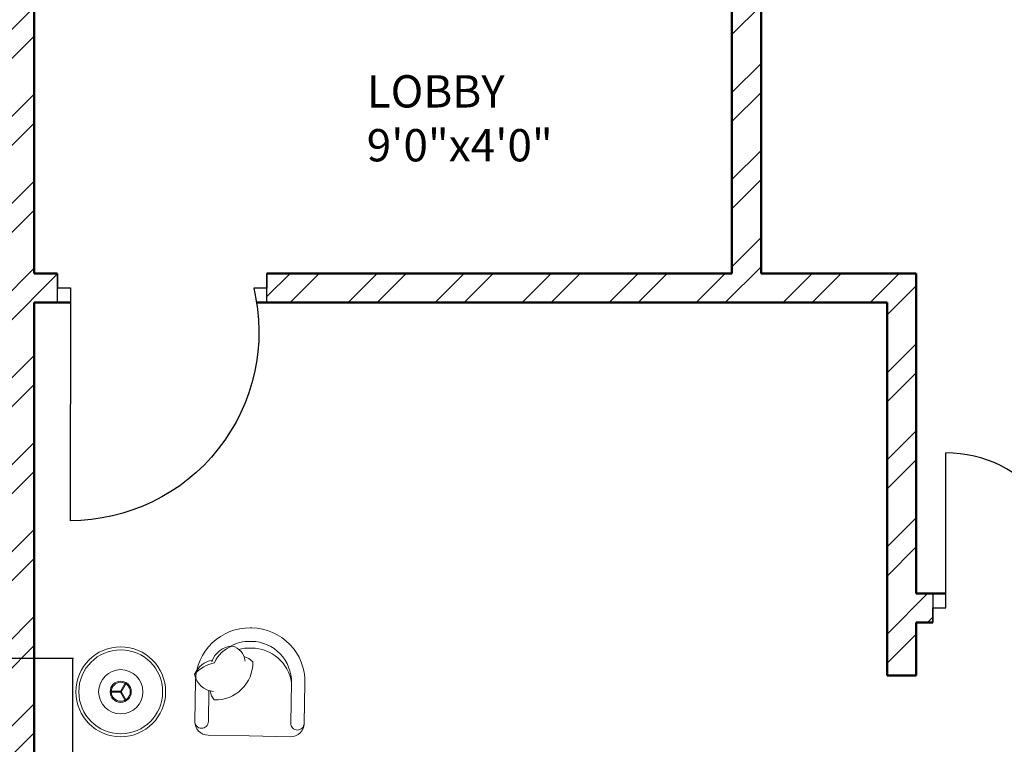
# Model space of a CAD drawing. Units: inches. Extents: x 963 to 2075, y 289 to 2657.
# Tile 54 of 98: x 1511 to 1663, y 1803 to 1915. Entities that reach past the tile are written whole.
import ezdxf

# ---------------------------------------------------------------- set-up
doc = ezdxf.new("R2010")
doc.units = ezdxf.units.IN
for name, color, linetype, lineweight in [('A-ANNO-DIMS', 2, 'Continuous', 18), ('A-AREA-IDEN', 7, 'Continuous', 18), ('A-DOOR', 4, 'Continuous', 25), ('A-FURN', 8, 'Continuous', 18), ('A-WALL', 7, 'Continuous', 50), ('A-WALL-PATT', 8, 'Continuous', 13)]:
    doc.layers.add(name, color=color, linetype=linetype, lineweight=lineweight)
doc.styles.get("Standard").update_dxf_attribs({"font": 'arial.ttf'})
doc.dimstyles.get("Standard").update_dxf_attribs({"dimtxt": 0.18, "dimasz": 0.18, "dimexe": 0.18, "dimexo": 0.0625, "dimgap": 0.09, "dimtad": 0, "dimtih": 1, "dimtoh": 1, "dimdec": 4, "dimzin": 0, "dimdsep": 46, "dimtxsty": 'Standard', "dimcen": 0.09, "dimadec": 0, "dimazin": 0, "dimtfac": 1, "dimtdec": 4, "dimtofl": 0, "dimtmove": 0, "dimatfit": 3, "dimfxl": 1, "dimtolj": 1, "dimtzin": 0, "dimarcsym": 0})

# ---------------------------------------------------------------- blocks, each defined once
blk = doc.blocks.new('ARMCHAIR-B')
at = {"ltscale": 0.03}
blk.add_lwpolyline([(8.89, -0.24), (2.51, -0.24, -0.414214), (0.42, 1.85), (0.42, 8.12, -0.414214), (8.78, 16.48), (8.89, 16.48), (8.99, 16.48, -0.414214), (17.35, 8.12), (17.35, 1.85, -0.414214), (15.26, -0.24), (8.89, -0.24)], format="xyb", dxfattribs=at)
for points in [[(2.51, 8.12, -0.414214), (8.78, 14.39), (8.89, 14.39)], [(12.1, 13.56, 0.130591), (8.99, 14.39), (8.89, 14.39)], [(2.51, 8.12, -0.372719), (8.78, 13.35), (8.89, 13.35)], [(10.77, 13.12, 0.072384), (8.99, 13.35), (8.89, 13.35)], [(14.89, 11.12, 0.306663), (11.77, 13.61, 0.30633), (9.74, 11.33, -0.872847)], [(17.52, 9.18, 0.14773), (14.47, 10.97, 0.213343), (11.77, 13.61, 0.178662)], [(15.05, 6.61, -0.165541), (14.41, 5.23, -0.425989), (8.54, 11.21, -0.121523), (9.93, 12.04, 7.115464)], [(14.53, 6.54, 0.356772), (17.52, 9.18, 0.249542), (14.81, 11.35, -9.61688)], [(2.51, 8.12), (2.51, 1.85, -0.414214), (1.47, 0.81), (1.47, 0.81, -0.414214), (0.42, 1.85)], [(15.26, 6.66), (15.26, 1.85, 0.414214), (16.31, 0.81), (16.31, 0.81, 0.414214), (17.35, 1.85)]]:
    blk.add_lwpolyline(points, format="xyb")
blk = doc.blocks.new('DOOR-3')
for p, q in [((2, 2.25), (2, 38.25)), ((0, 4.5), (0, 0)), ((32.39, 4.5), (32.39, 0)), ((0, 0), (0, 2.25)), ((0, 2.25), (2, 2.25)), ((32.39, 2.25), (30.39, 2.25)), ((32.39, 0), (32.39, 2.25))]:
    blk.add_line(p, q)
blk.add_arc((2, 9.06), 29.19, 346.5105, 90)
blk = doc.blocks.new('*D28')
at = {"layer": 'A-ANNO-DIMS', "color": 0, "lineweight": -2, "transparency": 16777216}
for p, q in [((1506.73, 1816.32), (1519.01, 1816.32)), ((1518.83, 1816.14), (1518.83, 1775.94)), ((1518.83, 1735.38), (1518.83, 1775.58)), ((1506.73, 1735.2), (1519.01, 1735.2))]:
    blk.add_line(p, q, dxfattribs=at)
at = {"layer": 'A-ANNO-DIMS', "color": 0, "transparency": 16777216}
for points in [[(1518.8, 1816.14), (1518.86, 1816.14), (1518.83, 1816.32)], [(1518.8, 1735.38), (1518.86, 1735.38), (1518.83, 1735.2)]]:
    blk.add_solid(points, dxfattribs=at)
at = {"layer": 'Defpoints', "color": 0, "transparency": 16777216}
for p in [(1506.66, 1816.32), (1518.83, 1816.32), (1506.66, 1735.2)]:
    blk.add_point(p, dxfattribs=at)
at = {"layer": 'A-ANNO-DIMS', "color": 0, "transparency": 16777216, "insert": (1518.83, 1775.76), "char_height": 0.18, "attachment_point": 5}
blk.add_mtext('\\A1;3-SEAT SOFA 81 TYP.', dxfattribs=at)

msp = doc.modelspace()

# ---------------------------------------------------------------- hatches: boundary and pattern name
at = {"layer": 'A-WALL-PATT'}
h = msp.add_hatch(dxfattribs=at)
h.set_pattern_fill('ANSI32', color=256)
h.paths.add_polyline_path([(1473.61, 2163.07), (1473.61, 2165.32), (1376.42, 2165.32), (1376.42, 2227.98), (1371.92, 2227.98), (1371.92, 2214.82), (1368.41, 2214.82), (1368.41, 2210.32), (1371.92, 2210.32), (1371.92, 2160.82), (1395.92, 2160.82), (1395.92, 2090.32), (1217.34, 2090.32), (1217.34, 2085.82), (1395.92, 2085.82), (1458.92, 2085.82), (1458.92, 2108.32), (1454.42, 2108.32), (1454.42, 2090.32), (1400.42, 2090.32), (1400.42, 2160.82), (1473.61, 2160.82)])
h.paths.add_polyline_path([(1649.42, 2210.32), (1653.23, 2210.32), (1653.23, 2214.82), (1649.42, 2214.82), (1649.42, 2227.98), (1644.92, 2227.98), (1644.92, 2165.32), (1550.1, 2165.32), (1550.1, 2160.82), (1620.92, 2160.82), (1620.92, 2112.82), (1555.45, 2112.82), (1555.45, 2108.32), (1584.33, 2108.32), (1584.33, 2084.92), (1588.83, 2084.92), (1588.83, 2108.32), (1625.42, 2108.32), (1667.95, 2108.32), (1667.95, 2022.67), (1588.83, 2022.67), (1588.83, 2047.41), (1584.33, 2047.41), (1584.33, 1996), (1588.83, 1996), (1588.83, 2018.32), (1667.95, 2018.17), (1667.95, 1928.32), (1625.42, 1928.32), (1625.42, 1923.82), (1672.45, 1923.82), (1672.45, 1928.32), (1672.45, 1946.66), (1785.45, 1946.66), (1785.45, 1951.16), (1743.03, 1951.16), (1743.03, 2017.92), (1841.42, 2017.92), (1841.42, 2014.77), (1845.92, 2014.77), (1845.92, 2017.92), (1905.92, 2017.92), (1905.92, 1987.51), (1910.42, 1987.51), (1910.42, 2022.42), (1910.42, 2068.52), (1905.92, 2068.52), (1905.92, 2022.42), (1845.92, 2022.42), (1845.92, 2025.85), (1843.67, 2025.85), (1841.42, 2025.85), (1841.42, 2022.42), (1743.03, 2022.42), (1743.03, 2084.03), (1768.45, 2084.03), (1785.45, 2084.03), (1785.45, 2088.53), (1672.45, 2088.53), (1672.45, 2112.82), (1667.95, 2112.82), (1625.42, 2112.82), (1625.42, 2160.82), (1649.42, 2160.82)])
h.paths.add_polyline_path([(1672.45, 2084.03), (1738.53, 2084.03), (1738.53, 1951.16), (1672.45, 1951.16)], flags=16)
h.paths.add_polyline_path([(1672.45, 2084.03), (1738.53, 2084.03), (1705.49, 2017.6)], flags=0)
h.paths.add_polyline_path([(1262.77, 2085.82), (1258.27, 2085.82), (1258.27, 2023.28), (1184.42, 2023.28), (1184.42, 2018.78), (1258.27, 2018.78), (1258.27, 1950.82), (1262.77, 1950.82)])
h.paths.add_polyline_path([(1312.27, 2085.82), (1307.77, 2085.82), (1307.77, 1950.82), (1312.27, 1950.82)])
h.paths.add_polyline_path([(1458.92, 1950.82), (1395.92, 1950.82), (1216.57, 1950.82), (1216.57, 1946.32), (1346.42, 1946.32), (1395.92, 1946.32), (1395.92, 1875.82), (1371.92, 1875.82), (1371.92, 1826.32), (1368.93, 1826.32), (1368.93, 1821.82), (1371.92, 1821.82), (1371.92, 1813.62), (1376.42, 1813.62), (1376.42, 1871.32), (1474.5, 1871.32), (1474.5, 1873.57), (1474.5, 1875.82), (1400.42, 1875.82), (1400.42, 1946.32), (1454.42, 1946.32), (1454.42, 1928.32), (1458.92, 1928.32)])
h.paths.add_polyline_path([(1184.42, 2120.78), (1167.92, 2120.78), (1167.92, 2134.81), (1165.67, 2134.81), (1163.42, 2134.81), (1163.42, 2120.78), (1119.92, 2120.78), (1119.92, 2098.1), (1124.42, 2098.1), (1124.42, 2116.28), (1167.92, 2116.28), (1179.92, 2116.28), (1179.92, 2045.92), (1184.42, 2045.92), (1184.42, 2090.32), (1184.42, 2116.28)])
h.paths.add_polyline_path([(1124.42, 2018.78), (1179.92, 2018.78), (1179.92, 2016.29), (1184.42, 2016.29), (1184.42, 2023.28), (1184.42, 2026.59), (1182.17, 2026.59), (1179.92, 2026.59), (1179.92, 2023.28), (1124.42, 2023.28), (1124.42, 2074.1), (1119.92, 2074.1), (1119.92, 2018.78), (1119.92, 1979.63), (1124.42, 1979.63)])
h.paths.add_polyline_path([(1184.42, 1925.78), (1184.42, 1946.32), (1184.42, 1996.07), (1182.17, 1996.07), (1179.92, 1996.07), (1179.92, 1925.78), (1124.42, 1925.78), (1124.42, 1955.63), (1119.92, 1955.5), (1119.92, 1921.28), (1158.92, 1921.28), (1158.92, 1909.98), (1163.42, 1909.98), (1163.42, 1921.28), (1184.42, 1921.28)])
h.paths.add_polyline_path([(1341.45, 1826.32), (1163.42, 1826.32), (1163.42, 1849.98), (1158.92, 1849.98), (1158.92, 1821.82), (1158.92, 1804.03), (1163.42, 1804.03), (1163.42, 1821.82), (1341.45, 1821.82)])
h.paths.add_polyline_path([(1222.98, 1713.82), (1163.42, 1713.82), (1163.42, 1744.03), (1161.17, 1744.03), (1158.92, 1744.03), (1158.92, 1713.82), (1119.92, 1713.82), (1119.92, 1694.65), (1124.42, 1694.65), (1124.42, 1709.32), (1158.92, 1709.32), (1222.98, 1709.32)])
h.paths.add_polyline_path([(1328.42, 1713.82), (1252.04, 1713.82), (1252.04, 1711.57), (1252.04, 1709.32), (1256.42, 1709.32), (1256.42, 1547.32), (1232.94, 1547.32), (1232.94, 1545.07), (1232.94, 1542.82), (1292.42, 1542.82), (1292.42, 1527.63), (1296.92, 1527.63), (1296.92, 1542.82), (1299.46, 1542.82), (1299.46, 1547.32), (1260.92, 1547.32), (1260.92, 1658.32), (1343.66, 1658.32), (1343.66, 1660.57), (1343.66, 1662.82), (1328.42, 1662.82), (1328.42, 1676.59), (1327.4, 1676.59), (1323.92, 1676.59), (1323.92, 1662.82), (1260.92, 1662.82), (1260.92, 1709.32), (1323.92, 1709.32), (1323.92, 1699.85), (1328.42, 1699.85)])
h.paths.add_polyline_path([(1649.42, 1875.82), (1625.42, 1875.82), (1625.42, 1928.32), (1620.92, 1928.32), (1588.83, 1928.32), (1588.83, 1950.59), (1584.33, 1950.59), (1584.33, 1928.32), (1555.45, 1928.32), (1555.45, 1923.82), (1620.92, 1923.82), (1620.92, 1875.82), (1548.95, 1875.82), (1548.95, 1873.57), (1548.95, 1871.32), (1644.92, 1871.32), (1644.92, 1813.62), (1649.42, 1813.62), (1649.42, 1821.82), (1652.04, 1821.82), (1652.04, 1824.07), (1652.04, 1826.32), (1649.42, 1826.32)])
h.paths.add_polyline_path([(1512.92, 1871.32), (1516.48, 1871.32), (1516.48, 1875.82), (1512.92, 1875.82), (1512.92, 1923.82), (1512.92, 1928.32), (1512.92, 1930.83), (1508.42, 1930.83), (1508.42, 1875.82), (1504.41, 1875.82), (1504.41, 1871.32), (1508.42, 1871.32), (1508.42, 1713.82), (1376.42, 1713.82), (1376.42, 1743.32), (1371.92, 1743.32), (1371.92, 1709.32), (1371.92, 1706.01), (1376.42, 1706.01), (1376.42, 1709.32), (1508.42, 1709.32), (1508.42, 1547.32), (1501.87, 1547.32), (1501.87, 1542.82), (1508.42, 1542.82), (1508.42, 1482.82), (1508.42, 1436.32), (1512.92, 1436.32), (1512.92, 1542.82), (1519.32, 1542.82), (1519.32, 1545.07), (1519.32, 1547.32), (1512.92, 1547.32), (1512.92, 1709.32), (1644.92, 1709.32), (1644.92, 1707.55), (1649.42, 1707.55), (1649.42, 1709.32), (1649.42, 1743.32), (1644.92, 1743.32), (1644.92, 1713.82), (1512.92, 1713.82)])
h.paths.add_polyline_path([(1129.88, 1545.07), (1129.88, 1547.32), (1124.42, 1547.32), (1095.92, 1547.32), (1095.92, 1614.82), (1124.42, 1614.82), (1124.42, 1619.32), (1095.92, 1619.32), (1091.42, 1619.32), (1091.42, 1542.82), (1095.92, 1542.82), (1119.92, 1542.82), (1129.88, 1542.82)])
h.paths.add_polyline_path([(1208.42, 1542.82), (1211.74, 1542.82), (1211.74, 1547.32), (1198.85, 1547.32), (1198.85, 1542.82), (1203.92, 1542.82), (1203.92, 1478.32), (1208.42, 1478.32), (1296.92, 1478.32), (1296.92, 1503.63), (1292.42, 1503.63), (1292.42, 1482.82), (1208.42, 1482.82)])
h.paths.add_polyline_path([(1430.42, 1542.82), (1435.7, 1542.82), (1435.7, 1545.07), (1435.7, 1547.32), (1422.66, 1547.32), (1422.66, 1545.07), (1422.66, 1542.82), (1425.92, 1542.82), (1425.92, 1482.86), (1341.92, 1482.86), (1341.92, 1502.73), (1337.42, 1502.73), (1337.42, 1478.36), (1425.92, 1478.36), (1425.92, 1440.82), (1425.92, 1436.32), (1430.42, 1436.32)])
h.paths.add_polyline_path([(1698.48, 2004.26), (1727.69, 2004.26), (1727.69, 2022.92), (1698.48, 2022.92)], flags=8)

# ---------------------------------------------------------------- linework, layer by layer
at = {"layer": 'A-DOOR'}
for p, q in [((1654.04, 1824.07), (1654.04, 1848.07)), ((1652.04, 1826.32), (1652.04, 1821.82)), ((1652.04, 1821.82), (1652.04, 1824.07)), ((1652.04, 1824.07), (1654.04, 1824.07))]:
    msp.add_line(p, q, dxfattribs=at)
msp.add_arc((1654.04, 1828.99), 19.08, 345.0651, 90, dxfattribs=at)
at = {"layer": 'A-FURN', "ltscale": 0.03}
for p, q in [((1526.25, 1811.15), (1527.07, 1812.56)), ((1526.38, 1811.07), (1527.19, 1812.49)), ((1526.31, 1811.18), (1524.68, 1811.18)), ((1526.31, 1811.04), (1524.68, 1811.04)), ((1526.25, 1811.07), (1527.07, 1809.66)), ((1526.38, 1811.15), (1527.19, 1809.73))]:
    msp.add_line(p, q, dxfattribs=at)
for radius in [6.95, 3.42, 1.64, 1.47]:
    msp.add_circle((1526.31, 1811.11), radius, dxfattribs=at)
at = {"layer": 'A-FURN'}
msp.add_circle((1526.31, 1811.11), 6.49, dxfattribs=at)
at = {"layer": 'A-WALL'}
for p, q in [((1625.42, 1928.32), (1625.42, 1875.82)), ((1512.92, 1875.82), (1512.92, 1923.82)), ((1620.92, 1875.82), (1620.92, 1923.82)), ((1512.92, 1875.82), (1516.48, 1875.82)), ((1548.95, 1875.82), (1620.92, 1875.82)), ((1625.42, 1875.82), (1649.42, 1875.82)), ((1649.42, 1826.32), (1649.42, 1875.82)), ((1512.92, 1713.82), (1512.92, 1871.32)), ((1518.48, 1871.32), (1512.92, 1871.32)), ((1644.92, 1871.32), (1547.39, 1871.32)), ((1644.92, 1813.62), (1644.92, 1871.32)), ((1649.42, 1826.32), (1654.04, 1826.32)), ((1649.42, 1821.82), (1652.04, 1821.82)), ((1649.42, 1813.62), (1649.42, 1821.82)), ((1649.42, 1813.62), (1644.92, 1813.62))]:
    msp.add_line(p, q, dxfattribs=at)

# ---------------------------------------------------------------- block references
at = {"layer": 'A-DOOR', "extrusion": (0, 0, -1), "zscale": -1, "rotation": 180.057037802669}
msp.add_blockref('DOOR-3', (-1516.52, 1875.83), dxfattribs=at)
at = {"layer": 'A-FURN', "extrusion": (0, 0, -1), "zscale": -1, "rotation": 1.04008870694515}
msp.add_blockref('ARMCHAIR-B', (-1555.1, 1804.36), dxfattribs=at)

# ---------------------------------------------------------------- texts
at = {"layer": 'A-AREA-IDEN', "insert": (1564.39, 1906.49), "char_height": 5, "attachment_point": 1}
msp.add_mtext_dynamic_manual_height_columns('LOBBY\\P9\'0"x4\'0"', width=97.0875, gutter_width=12.5, heights=[0], dxfattribs=at)

# ---------------------------------------------------------------- dimensions: what is measured, and where the dimension line sits
at = {"layer": 'A-ANNO-DIMS'}
dim = msp.add_linear_dim(base=(1518.83, 1816.32), p1=(1506.66, 1735.2), p2=(1506.66, 1816.32), angle=90, text='3-SEAT SOFA <> TYP.', dimstyle='Standard', override={"dimdec": 0, "dimlfac": 1, "dimrnd": 0, "dimzin": 0, "dimdsep": 46, "dimlunit": 2}, dxfattribs=at)
dim.commit()
dim.dimension.update_dxf_attribs({"geometry": '*D28', "text_midpoint": (1518.83, 1775.76)})

doc.saveas('drawing.dxf')
